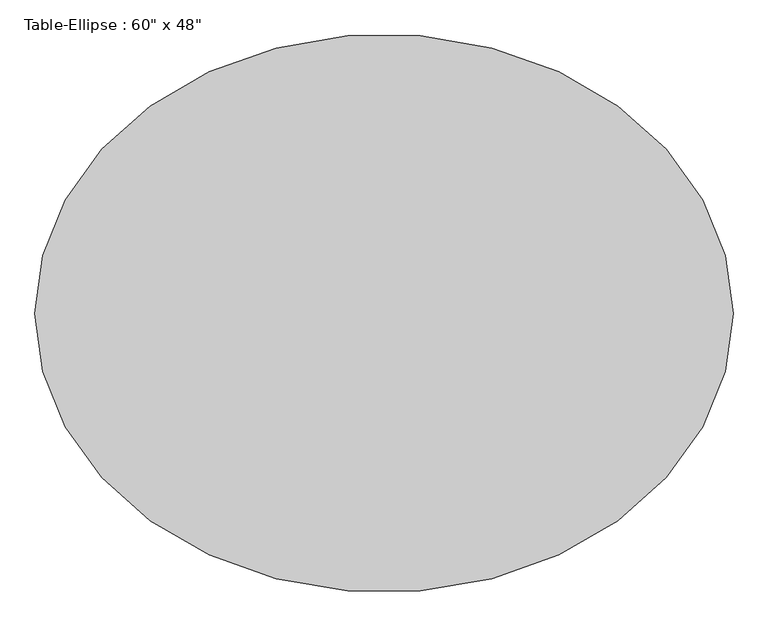
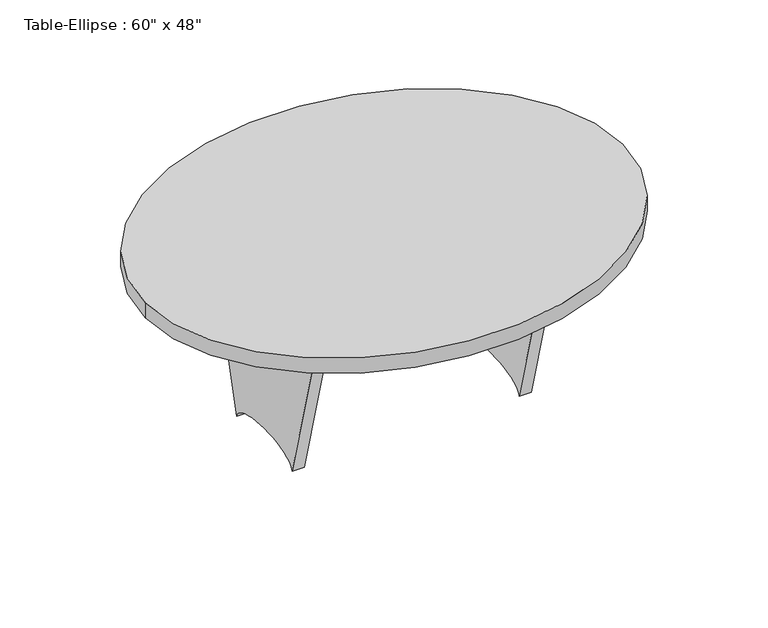
"""IFC4 building model written with IfcOpenShell, lengths in millimetres: furniture geometry."""

from ifc_helpers import new_model, si_unit, point, frame, origin, place, context, project, spatial, ellipse_curve, trimmed, source, transform, mapped, element, save
from ifc_brep_helpers import plane_surface, extruded_surface, advanced_brep


def furniture_cacb7300(model_context):
    return source(origin(), model_context, "Body", "AdvancedBrep", [
        advanced_brep(
        [(-342.9, 19.05, 558.8), (342.9, 19.05, 558.8), (342.9, 19.05, 372.5333333), (-342.9, 19.05, 372.5333333), (-342.9, -19.05, 558.8), (-342.9, -19.05, 372.5333333), (342.9, -19.05, 372.5333333), (342.9, -19.05, 558.8)],
        [
            (0, 1),
            (1, 2),
            (2, 3, ellipse_curve(frame((0.0, 19.05, 372.5333333), z_axis=(0.0, -1.0, 0.0), x_axis=(1.0, 0.0, 0.0)), 342.9, 101.6)),
            (3, 0),
            (4, 5),
            (5, 6, ellipse_curve(frame((0.0, -19.05, 372.5333333), z_axis=(0.0, 1.0, 0.0), x_axis=(1.0, 0.0, 0.0)), 342.9, 101.6)),
            (6, 7),
            (7, 4),
            (0, 4),
            (7, 1),
            (6, 2),
            (5, 3),
        ],
        [
            plane_surface(frame((-342.9, 19.05, 558.8), z_axis=(0.0, 1.0, 0.0), x_axis=(1.0, 0.0, 0.0))),
            plane_surface(frame((-342.9, -19.05, 558.8), z_axis=(0.0, -1.0, 0.0), x_axis=(-1.0, 0.0, 0.0))),
            plane_surface(frame((-342.9, 19.05, 558.8), z_axis=(0.0, 0.0, 1.0), x_axis=(0.0, -1.0, 0.0))),
            plane_surface(frame((342.9, 19.05, 558.8), z_axis=(1.0, 0.0, 0.0), x_axis=(0.0, -1.0, 0.0))),
            extruded_surface(trimmed(ellipse_curve(frame((0.0, -57.15, 372.5333333), z_axis=(0.0, -1.0, 0.0), x_axis=(1.0, 0.0, 0.0)), 342.9, 101.6), [point((342.9, -57.15, 372.5333333))], [point((-342.9, -57.15, 372.5333333))], True, "CARTESIAN"), (0.0, 38.099999999999994, 0.0), 38.099999999999994),
            plane_surface(frame((-342.9, 19.05, 372.5333333), z_axis=(-1.0, 0.0, 0.0), x_axis=(0.0, -1.0, 0.0))),
        ],
        [
            (0, [[1, 2, 3, 4]]),
            (1, [[5, 6, 7, 8]]),
            (2, [[-1, 9, -8, 10]]),
            (3, [[-2, -10, -7, 11]]),
            (4, [[-3, -11, -6, 12]]),
            (5, [[-4, -12, -5, -9]]),
        ],
    ),
        advanced_brep(
        [(381.0, 304.8, 558.8), (381.0, -304.8, 558.8), (381.0, -152.4, 0.0), (381.0, 152.4, 0.0), (342.9, 304.8, 558.8), (342.9, 152.4, 0.0), (342.9, -152.4, 0.0), (342.9, -304.8, 558.8)],
        [
            (0, 1),
            (1, 2),
            (2, 3, ellipse_curve(frame((381.0, 0.0, 0.0), z_axis=(-1.0, 0.0, 0.0), x_axis=(0.0, 1.0, 0.0)), 152.4, 50.8)),
            (3, 0),
            (4, 5),
            (5, 6, ellipse_curve(frame((342.9, 0.0, 0.0), z_axis=(1.0, 0.0, 0.0), x_axis=(0.0, 1.0, 0.0)), 152.4, 50.8)),
            (6, 7),
            (7, 4),
            (0, 4),
            (7, 1),
            (6, 2),
            (5, 3),
        ],
        [
            plane_surface(frame((381.0, -304.8, 558.8), z_axis=(1.0, 0.0, 0.0), x_axis=(0.0, -1.0, 0.0))),
            plane_surface(frame((342.9, -304.8, 558.8), z_axis=(-1.0, 0.0, 0.0), x_axis=(0.0, 1.0, 0.0))),
            plane_surface(frame((381.0, 304.8, 558.8), z_axis=(0.0, 0.0, 1.0), x_axis=(-1.0, 0.0, 0.0))),
            plane_surface(frame((381.0, -304.8, 558.8), z_axis=(0.0, -0.9647638212377304, -0.2631174057921153), x_axis=(-1.0, 0.0, 0.0))),
            extruded_surface(trimmed(ellipse_curve(frame((304.8, 0.0, 0.0), z_axis=(-1.0, 0.0, 0.0), x_axis=(0.0, 1.0, 0.0)), 152.4, 50.8), [point((304.8, -152.4, 0.0))], [point((304.8, 152.4, 0.0))], True, "CARTESIAN"), (38.099999999999966, 0.0, 0.0), 38.099999999999966),
            plane_surface(frame((381.0, 152.4, 0.0), z_axis=(0.0, 0.9647638212377352, -0.2631174057920975), x_axis=(-1.0, 0.0, 0.0))),
        ],
        [
            (0, [[1, 2, 3, 4]]),
            (1, [[5, 6, 7, 8]]),
            (2, [[-1, 9, -8, 10]]),
            (3, [[-2, -10, -7, 11]]),
            (4, [[-3, -11, -6, 12]]),
            (5, [[-4, -12, -5, -9]]),
        ],
    ),
        advanced_brep(
        [(-342.9, 304.8, 558.8), (-342.9, -304.8, 558.8), (-342.9, -152.4, 0.0), (-342.9, 152.4, 0.0), (-381.0, 304.8, 558.8), (-381.0, 152.4, 0.0), (-381.0, -152.4, 0.0), (-381.0, -304.8, 558.8)],
        [
            (0, 1),
            (1, 2),
            (2, 3, ellipse_curve(frame((-342.9, 0.0, 0.0), z_axis=(-1.0, 0.0, 0.0), x_axis=(0.0, 1.0, 0.0)), 152.4, 50.8)),
            (3, 0),
            (4, 5),
            (5, 6, ellipse_curve(frame((-381.0, 0.0, 0.0), z_axis=(1.0, 0.0, 0.0), x_axis=(0.0, 1.0, 0.0)), 152.4, 50.8)),
            (6, 7),
            (7, 4),
            (0, 4),
            (7, 1),
            (6, 2),
            (5, 3),
        ],
        [
            plane_surface(frame((-342.9, -304.8, 558.8), z_axis=(1.0, 0.0, 0.0), x_axis=(0.0, -1.0, 0.0))),
            plane_surface(frame((-381.0, -304.8, 558.8), z_axis=(-1.0, 0.0, 0.0), x_axis=(0.0, 1.0, 0.0))),
            plane_surface(frame((-342.9, 304.8, 558.8), z_axis=(0.0, 0.0, 1.0), x_axis=(-1.0, 0.0, 0.0))),
            plane_surface(frame((-342.9, -304.8, 558.8), z_axis=(0.0, -0.9647638212377301, -0.26311740579211657), x_axis=(-1.0, 0.0, 0.0))),
            extruded_surface(trimmed(ellipse_curve(frame((-419.1, 0.0, 0.0), z_axis=(-1.0, 0.0, 0.0), x_axis=(0.0, 1.0, 0.0)), 152.4, 50.8), [point((-419.1, -152.4, 0.0))], [point((-419.1, 152.4, 0.0))], True, "CARTESIAN"), (38.10000000000002, 0.0, 0.0), 38.10000000000002),
            plane_surface(frame((-342.9, 152.4, 0.0), z_axis=(0.0, 0.9647638212377332, -0.2631174057921053), x_axis=(-1.0, 0.0, 0.0))),
        ],
        [
            (0, [[1, 2, 3, 4]]),
            (1, [[5, 6, 7, 8]]),
            (2, [[-1, 9, -8, 10]]),
            (3, [[-2, -10, -7, 11]]),
            (4, [[-3, -11, -6, 12]]),
            (5, [[-4, -12, -5, -9]]),
        ],
    ),
        advanced_brep(
        [(-762.0, 0.0, 609.6), (762.0, 0.0, 609.6), (-762.0, 0.0, 558.8), (762.0, 0.0, 558.8)],
        [
            (0, 1, ellipse_curve(frame((0.0, 0.0, 609.6), z_axis=(0.0, 0.0, 1.0), x_axis=(1.0, 0.0, 0.0)), 762.0, 609.6)),
            (1, 0, ellipse_curve(frame((0.0, 0.0, 609.6), z_axis=(0.0, 0.0, 1.0), x_axis=(1.0, 0.0, 0.0)), 762.0, 609.6)),
            (2, 3, ellipse_curve(frame((0.0, 0.0, 558.8), z_axis=(0.0, 0.0, -1.0), x_axis=(1.0, 0.0, 0.0)), 762.0, 609.6)),
            (3, 2, ellipse_curve(frame((0.0, 0.0, 558.8), z_axis=(0.0, 0.0, -1.0), x_axis=(1.0, 0.0, 0.0)), 762.0, 609.6)),
            (0, 2),
            (3, 1),
        ],
        [
            plane_surface(frame((762.0, 0.0, 609.6), z_axis=(0.0, 0.0, 1.0), x_axis=(0.0, 1.0, 0.0))),
            plane_surface(frame((762.0, 0.0, 558.8), z_axis=(0.0, 0.0, -1.0), x_axis=(0.0, -1.0, 0.0))),
            extruded_surface(trimmed(ellipse_curve(frame((0.0, 0.0, 508.0), z_axis=(0.0, 0.0, 1.0), x_axis=(1.0, 0.0, 0.0)), 762.0, 609.6), [point((-762.0, 0.0, 508.0))], [point((762.0, 0.0, 508.0))], True, "CARTESIAN"), (0.0, 0.0, 50.799999999999955), 50.799999999999955),
            extruded_surface(trimmed(ellipse_curve(frame((0.0, 0.0, 508.0), z_axis=(0.0, 0.0, 1.0), x_axis=(1.0, 0.0, 0.0)), 762.0, 609.6), [point((762.0, 0.0, 508.0))], [point((-762.0, 0.0, 508.0))], True, "CARTESIAN"), (0.0, 0.0, 50.799999999999955), 50.799999999999955),
        ],
        [
            (0, [[1, 2]]),
            (1, [[3, 4]]),
            (2, [[-1, 5, -4, 6]]),
            (3, [[-2, -6, -3, -5]]),
        ],
    ),
    ])


if __name__ == "__main__":
    model = new_model("IFC4")
    model_context = context("Model", 3, world=origin())
    ifc_project = project(units=[si_unit("LENGTHUNIT", "METRE", prefix="MILLI")], contexts=[model_context])
    site = spatial("IfcSite", under=ifc_project)
    building = spatial("IfcBuilding", under=site)
    placement = place(None, origin())
    furniture_shape = furniture_cacb7300(model_context)
    element("IfcFurniture", 1, ObjectType="Table-Ellipse : 60\" x 48\"", at=placement, inside=building, context=model_context, shape_type="MappedRepresentation", body=[
        mapped(furniture_shape, transform((0.0, 0.0, 0.0), x_axis=(1.0, 0.0, 0.0), y_axis=(0.0, 1.0, 0.0), z_axis=(0.0, 0.0, 1.0))),
    ])
    save(model, "model.ifc")

# Revit data of these elements
# Type "Table-Ellipse : 60\" x 48\""
#   Assembly Code = "E2020200"
#   Half Width = 2' - 0"
#   Half Length = 2' - 6"
#   Height = 2' - 0"
#   Length = 5' - 0"
#   Width = 4' - 0"
#   Base Material = Birch
#   Top Material = Birch
#   Default Elevation = 0
# Element 1 (IfcFurniture, "Table-Ellipse : 60\" x 48\"")
#   Materials on its faces: "Birch"
# Materials
#   "Birch": class "Wood", colour RGB 224 178 126, transparency 0, Description = "Betula Alleghaniensis", Cost = 0
